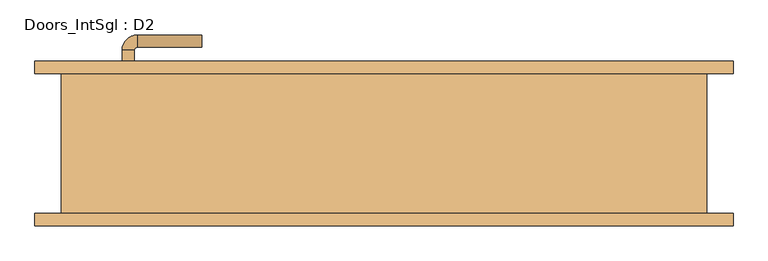
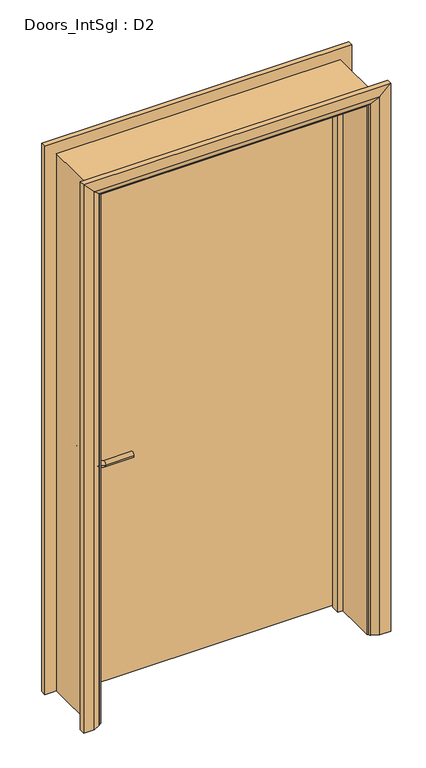
"""IFC4 building model written with IfcOpenShell, lengths in millimetres: door geometry, Doors_IntSgl : D2."""

from ifc_helpers import new_model, si_unit, point, frame, frame_2d, origin, place, context, project, spatial, polyline, circle_curve, ellipse_curve, trimmed, segment, composite_curve, outline, extrude, faceted_brep, source, transform, mapped, element, save
from ifc_brep_helpers import plane_surface, cylinder_surface, revolved_surface, advanced_brep


def doors_intsgl_d2_1027b9ee(model_context):
    return source(origin(), model_context, "Body", "SolidModel", [
        advanced_brep(
        [(-426.4, 68.3, 900.0), (-406.4, 68.3, 900.0), (-406.4, 38.3, 900.0), (-426.4, 38.3, 900.0), (-401.4, 33.3, 900.0), (-401.4, 13.3, 900.0), (-296.4, 13.3, 900.0), (-296.4, 33.3, 900.0)],
        [
            (0, 1, circle_curve(frame((-416.4, 68.3, 900.0), z_axis=(0.0, 1.0, 0.0), x_axis=(1.0, 0.0, 0.0)), 10.0)),
            (1, 0, circle_curve(frame((-416.4, 68.3, 900.0), z_axis=(0.0, 1.0, 0.0), x_axis=(1.0, 0.0, 0.0)), 10.0)),
            (1, 2),
            (2, 3, circle_curve(frame((-416.4, 38.3, 900.0), z_axis=(0.0, 1.0, 0.0), x_axis=(1.0, 0.0, 0.0)), 10.0)),
            (3, 0),
            (3, 2, circle_curve(frame((-416.4, 38.3, 900.0), z_axis=(0.0, 1.0, 0.0), x_axis=(1.0, 0.0, 0.0)), 10.0)),
            (4, 5, circle_curve(frame((-401.4, 23.3, 900.0), z_axis=(-1.0, 0.0, 0.0), x_axis=(0.0, 1.0, 0.0)), 10.0)),
            (5, 3, circle_curve(frame((-401.4, 38.3, 900.0), z_axis=(0.0, 0.0, -1.0), x_axis=(-1.0, 0.0, 0.0)), 25.0)),
            (2, 4, circle_curve(frame((-401.4, 38.3, 900.0), z_axis=(0.0, 0.0, 1.0), x_axis=(-1.0, 0.0, 0.0)), 5.0)),
            (5, 4, circle_curve(frame((-401.4, 23.3, 900.0), z_axis=(-1.0, 0.0, 0.0), x_axis=(0.0, 1.0, 0.0)), 10.0)),
            (6, 7, circle_curve(frame((-296.4, 23.3, 900.0), z_axis=(1.0, 0.0, 0.0), x_axis=(0.0, 1.0, 0.0)), 10.0)),
            (7, 6, circle_curve(frame((-296.4, 23.3, 900.0), z_axis=(1.0, 0.0, 0.0), x_axis=(0.0, 1.0, 0.0)), 10.0)),
            (4, 7),
            (6, 5),
        ],
        [
            plane_surface(frame((-416.4, 68.3, 900.0), z_axis=(0.0, 1.0, 0.0), x_axis=(0.0, 0.0, 1.0))),
            cylinder_surface(frame((-416.4, 68.3, 900.0), z_axis=(0.0, 1.0, 0.0), x_axis=(1.0, 0.0, 0.0)), 10.0),
            revolved_surface(trimmed(ellipse_curve(frame((-416.4, 38.3, 900.0), z_axis=(0.0, -1.0, 0.0), x_axis=(1.0, 0.0, 0.0)), 10.0, 10.0), [point((-426.4, 38.3, 900.0))], [point((-406.4, 38.3, 900.0))], True, "CARTESIAN"), (-401.4, 38.3, 900.0), (0.0, 0.0, -1.0)),
            revolved_surface(trimmed(ellipse_curve(frame((-416.4, 38.3, 900.0), z_axis=(0.0, -1.0, 0.0), x_axis=(1.0, 0.0, 0.0)), 10.0, 10.0), [point((-406.4, 38.3, 900.0))], [point((-426.4, 38.3, 900.0))], True, "CARTESIAN"), (-401.4, 38.3, 900.0), (0.0, 0.0, -1.0)),
            plane_surface(frame((-296.4, 23.3, 900.0), z_axis=(1.0, 0.0, 0.0), x_axis=(0.0, 0.0, 1.0))),
            cylinder_surface(frame((-401.4, 23.3, 900.0), z_axis=(-1.0, 0.0, 0.0), x_axis=(0.0, 1.0, 0.0)), 10.0),
        ],
        [
            (0, [[1, 2]]),
            (1, [[3, 4, 5, -2]]),
            (1, [[-5, 6, -3, -1]]),
            (2, [[7, 8, -4, 9]]),
            (3, [[10, -9, -6, -8]]),
            (4, [[11, 12]]),
            (5, [[13, -11, 14, -7]]),
            (5, [[-14, -12, -13, -10]]),
        ],
    ),
        extrude(outline(composite_curve([segment(trimmed(circle_curve(frame_2d((900.0, -418.9)), 30.0), [point((900.0, -448.9))], [point((900.0, -388.9))], False, "CARTESIAN"), True, "CONTINUOUS"), segment(trimmed(circle_curve(frame_2d((900.0, -418.9)), 30.0), [point((900.0, -388.9))], [point((900.0, -448.9))], False, "CARTESIAN"), True, "CONTINUOUS")], self_intersect=False)), frame((0.0, 68.3, 0.0), z_axis=(0.0, 1.0, 0.0), x_axis=(0.0, 0.0, 1.0)), (0.0, 0.0, 1.0), 8.0),
        advanced_brep(
        [(-426.4, 122.3, 900.0), (-406.4, 122.3, 900.0), (-426.4, 152.3, 900.0), (-406.4, 152.3, 900.0), (-401.4, 157.3, 900.0), (-401.4, 177.3, 900.0), (-296.4, 177.3, 900.0), (-296.4, 157.3, 900.0)],
        [
            (0, 1, circle_curve(frame((-416.4, 122.3, 900.0), z_axis=(0.0, -1.0, 0.0), x_axis=(1.0, 0.0, 0.0)), 10.0)),
            (1, 0, circle_curve(frame((-416.4, 122.3, 900.0), z_axis=(0.0, -1.0, 0.0), x_axis=(1.0, 0.0, 0.0)), 10.0)),
            (0, 2),
            (2, 3, circle_curve(frame((-416.4, 152.3, 900.0), z_axis=(0.0, -1.0, 0.0), x_axis=(1.0, 0.0, 0.0)), 10.0)),
            (3, 1),
            (3, 2, circle_curve(frame((-416.4, 152.3, 900.0), z_axis=(0.0, -1.0, 0.0), x_axis=(1.0, 0.0, 0.0)), 10.0)),
            (4, 3, circle_curve(frame((-401.4, 152.3, 900.0), z_axis=(0.0, 0.0, 1.0), x_axis=(-1.0, 0.0, 0.0)), 5.0)),
            (2, 5, circle_curve(frame((-401.4, 152.3, 900.0), z_axis=(0.0, 0.0, -1.0), x_axis=(-1.0, 0.0, 0.0)), 25.0)),
            (5, 4, circle_curve(frame((-401.4, 167.3, 900.0), z_axis=(-1.0, 0.0, 0.0), x_axis=(0.0, -1.0, 0.0)), 10.0)),
            (4, 5, circle_curve(frame((-401.4, 167.3, 900.0), z_axis=(-1.0, 0.0, 0.0), x_axis=(0.0, -1.0, 0.0)), 10.0)),
            (6, 7, circle_curve(frame((-296.4, 167.3, 900.0), z_axis=(1.0, 0.0, 0.0), x_axis=(0.0, -1.0, 0.0)), 10.0)),
            (7, 6, circle_curve(frame((-296.4, 167.3, 900.0), z_axis=(1.0, 0.0, 0.0), x_axis=(0.0, -1.0, 0.0)), 10.0)),
            (5, 6),
            (7, 4),
        ],
        [
            plane_surface(frame((-416.4, 122.3, 900.0), z_axis=(0.0, -1.0, 0.0), x_axis=(0.0, 0.0, 1.0))),
            cylinder_surface(frame((-416.4, 122.3, 900.0), z_axis=(0.0, -1.0, 0.0), x_axis=(1.0, 0.0, 0.0)), 10.0),
            revolved_surface(trimmed(ellipse_curve(frame((-416.4, 152.3, 900.0), z_axis=(0.0, -1.0, 0.0), x_axis=(1.0, 0.0, 0.0)), 10.0, 10.0), [point((-426.4, 152.3, 900.0))], [point((-406.4, 152.3, 900.0))], True, "CARTESIAN"), (-401.4, 152.3, 900.0), (0.0, 0.0, -1.0)),
            revolved_surface(trimmed(ellipse_curve(frame((-416.4, 152.3, 900.0), z_axis=(0.0, -1.0, 0.0), x_axis=(1.0, 0.0, 0.0)), 10.0, 10.0), [point((-406.4, 152.3, 900.0))], [point((-426.4, 152.3, 900.0))], True, "CARTESIAN"), (-401.4, 152.3, 900.0), (0.0, 0.0, -1.0)),
            plane_surface(frame((-296.4, 167.3, 900.0), z_axis=(1.0, 0.0, 0.0), x_axis=(0.0, 0.0, 1.0))),
            cylinder_surface(frame((-401.4, 167.3, 900.0), z_axis=(-1.0, 0.0, 0.0), x_axis=(0.0, -1.0, 0.0)), 10.0),
        ],
        [
            (0, [[1, 2]]),
            (1, [[-1, 3, 4, 5]]),
            (1, [[-2, -5, 6, -3]]),
            (2, [[7, -4, 8, 9]]),
            (3, [[-8, -6, -7, 10]]),
            (4, [[11, 12]]),
            (5, [[-9, 13, -12, 14]]),
            (5, [[-10, -14, -11, -13]]),
        ],
    ),
        extrude(outline(composite_curve([segment(trimmed(circle_curve(frame_2d((900.0, -418.9)), 30.0), [point((900.0, -448.9))], [point((900.0, -388.9))], False, "CARTESIAN"), True, "CONTINUOUS"), segment(trimmed(circle_curve(frame_2d((900.0, -418.9)), 30.0), [point((900.0, -388.9))], [point((900.0, -448.9))], False, "CARTESIAN"), True, "CONTINUOUS")], self_intersect=False)), frame((0.0, 114.3, 0.0), z_axis=(0.0, 1.0, 0.0), x_axis=(0.0, 0.0, 1.0)), (0.0, 0.0, 1.0), 8.0),
        extrude(outline(polyline([(491.4, 76.3), (-491.4, 76.3), (-491.4, 114.3), (491.4, 114.3), (491.4, 76.3)])), frame((0.0, 0.0, 8.0), z_axis=(0.0, 0.0, 1.0), x_axis=(1.0, 0.0, 0.0)), (0.0, 0.0, 1.0), 2060.0),
        advanced_brep(
        [(568.4, 134.3, 0.0), (568.4, 114.3, 0.0), (498.4, 114.3, 0.0), (502.4, 120.3, 0.0), (528.4, 134.3, 0.0), (568.4, 134.3, 2145.0), (568.4, 114.3, 2145.0), (-568.4, 114.3, 2145.0), (-568.4, 114.3, 0.0), (-498.4, 114.3, 0.0), (-498.4, 114.3, 2075.0), (498.4, 114.3, 2075.0), (502.4, 120.3, 2079.0), (528.4, 134.3, 2105.0), (-528.4, 134.3, 2105.0), (-528.4, 134.3, 0.0), (-568.4, 134.3, 0.0), (-568.4, 134.3, 2145.0), (-502.4, 120.3, 0.0), (-502.4, 120.3, 2079.0)],
        [
            (0, 1),
            (1, 2),
            (2, 3, circle_curve(frame((506.4, 113.3, 0.0), z_axis=(0.0, 0.0, -1.0), x_axis=(1.0, 0.0, 0.0)), 8.0622577)),
            (3, 4),
            (4, 0),
            (0, 5),
            (5, 6),
            (6, 1),
            (6, 7),
            (7, 8),
            (8, 9),
            (9, 10),
            (10, 11),
            (11, 2),
            (11, 12, ellipse_curve(frame((506.4, 113.3, 2083.0), z_axis=(0.7071067811865475, 0.0, -0.7071067811865475), x_axis=(-0.7071067811865474, 0.0, -0.7071067811865476)), 11.4017543, 8.0622577)),
            (12, 3),
            (12, 13),
            (13, 4),
            (13, 14),
            (14, 15),
            (15, 16),
            (16, 17),
            (17, 5),
            (7, 17),
            (16, 8),
            (15, 18),
            (18, 9, circle_curve(frame((-506.4, 113.3, 0.0), z_axis=(0.0, 0.0, -1.0), x_axis=(-1.0, 0.0, 0.0)), 8.0622577)),
            (19, 10, ellipse_curve(frame((-506.4, 113.3, 2083.0), z_axis=(-0.7071067811865475, 0.0, -0.7071067811865475), x_axis=(-0.7071067811865474, 0.0, 0.7071067811865476)), 11.4017543, 8.0622577)),
            (18, 19),
            (14, 19),
            (19, 12),
        ],
        [
            plane_surface(frame((498.4, 114.3, 0.0), z_axis=(0.0, 0.0, -1.0), x_axis=(0.0, -1.0, 0.0))),
            plane_surface(frame((568.4, 134.3, 0.0), z_axis=(1.0, 0.0, 0.0), x_axis=(0.0, 0.0, 1.0))),
            plane_surface(frame((568.4, 114.3, 0.0), z_axis=(0.0, -1.0, 0.0), x_axis=(0.0, 0.0, 1.0))),
            cylinder_surface(frame((506.4, 113.3, 0.0), z_axis=(0.0, 0.0, -1.0), x_axis=(1.0, 0.0, 0.0)), 8.0622577),
            plane_surface(frame((502.4, 120.3, 0.0), z_axis=(-0.4740998230350126, 0.880471099922178, 0.0), x_axis=(0.0, 0.0, 1.0))),
            plane_surface(frame((528.4, 134.3, 0.0), z_axis=(0.0, 1.0, 0.0), x_axis=(0.0, 0.0, 1.0))),
            plane_surface(frame((-568.4, 134.3, 2145.0), z_axis=(-1.0, 0.0, 0.0), x_axis=(0.0, 0.0, -1.0))),
            plane_surface(frame((-498.4, 114.3, 0.0), z_axis=(0.0, 0.0, -1.0), x_axis=(0.0, -1.0, 0.0))),
            cylinder_surface(frame((-506.4, 113.3, 2075.0), z_axis=(0.0, 0.0, 1.0), x_axis=(-1.0, 0.0, 0.0)), 8.0622577),
            plane_surface(frame((-502.4, 120.3, 2079.0), z_axis=(0.47409982303501824, 0.8804710999221749, 0.0), x_axis=(0.0, 0.0, -1.0))),
            plane_surface(frame((568.4, 134.3, 2145.0), z_axis=(0.0, 0.0, 1.0), x_axis=(-1.0, 0.0, 0.0))),
            cylinder_surface(frame((498.4, 113.3, 2083.0), z_axis=(1.0, 0.0, 0.0), x_axis=(0.0, 0.0, 1.0)), 8.0622577),
            plane_surface(frame((502.4, 120.3, 2079.0), z_axis=(0.0, 0.8804710999221764, -0.4740998230350154), x_axis=(-1.0, 0.0, 0.0))),
        ],
        [
            (0, [[1, 2, 3, 4, 5]]),
            (1, [[-1, 6, 7, 8]]),
            (2, [[-2, -8, 9, 10, 11, 12, 13, 14]]),
            (3, [[-3, -14, 15, 16]]),
            (4, [[-4, -16, 17, 18]]),
            (5, [[-5, -18, 19, 20, 21, 22, 23, -6]]),
            (6, [[24, -22, 25, -10]]),
            (7, [[-21, 26, 27, -11, -25]]),
            (8, [[28, -12, -27, 29]]),
            (9, [[30, -29, -26, -20]]),
            (10, [[-7, -23, -24, -9]]),
            (11, [[-15, -13, -28, 31]]),
            (12, [[-17, -31, -30, -19]]),
        ],
    ),
        extrude(outline(polyline([(0.0, -493.4), (0.0, -474.4), (2051.0, -474.4), (2051.0, 474.4), (0.0, 474.4), (0.0, 493.4), (2070.0, 493.4), (2070.0, -493.4), (0.0, -493.4)])), frame((0.0, 42.3, 0.0), z_axis=(0.0, 1.0, 0.0), x_axis=(0.0, 0.0, 1.0)), (0.0, 0.0, 1.0), 32.0),
        advanced_brep(
        [(-568.4, -134.3, 0.0), (-568.4, -114.3, 0.0), (-498.4, -114.3, 0.0), (-502.4, -120.3, 0.0), (-528.4, -134.3, 0.0), (-568.4, -134.3, 2145.0), (-568.4, -114.3, 2145.0), (-498.4, -114.3, 2075.0), (-502.4, -120.3, 2079.0), (-528.4, -134.3, 2105.0), (568.4, -134.3, 0.0), (528.4, -134.3, 0.0), (502.4, -120.3, 0.0), (498.4, -114.3, 0.0), (568.4, -114.3, 0.0), (568.4, -134.3, 2145.0), (528.4, -134.3, 2105.0), (502.4, -120.3, 2079.0), (498.4, -114.3, 2075.0), (568.4, -114.3, 2145.0)],
        [
            (0, 1),
            (1, 2),
            (2, 3, circle_curve(frame((-506.4, -113.3, 0.0), z_axis=(0.0, 0.0, -1.0), x_axis=(-1.0, 0.0, 0.0)), 8.0622577)),
            (3, 4),
            (4, 0),
            (0, 5),
            (5, 6),
            (6, 1),
            (6, 7),
            (7, 2),
            (7, 8, ellipse_curve(frame((-506.4, -113.3, 2083.0), z_axis=(-0.7071067811865475, 0.0, -0.7071067811865475), x_axis=(0.7071067811865474, 0.0, -0.7071067811865476)), 11.4017543, 8.0622577)),
            (8, 3),
            (8, 9),
            (9, 4),
            (9, 5),
            (10, 11),
            (11, 12),
            (12, 13, circle_curve(frame((506.4, -113.3, 0.0), z_axis=(0.0, 0.0, -1.0), x_axis=(1.0, 0.0, 0.0)), 8.0622577)),
            (13, 14),
            (14, 10),
            (15, 16),
            (16, 11),
            (10, 15),
            (16, 17),
            (17, 12),
            (17, 18, ellipse_curve(frame((506.4, -113.3, 2083.0), z_axis=(0.7071067811865475, 0.0, -0.7071067811865475), x_axis=(0.7071067811865474, 0.0, 0.7071067811865476)), 11.4017543, 8.0622577)),
            (18, 13),
            (18, 19),
            (19, 14),
            (19, 15),
            (5, 15),
            (19, 6),
            (18, 7),
            (17, 8),
            (16, 9),
        ],
        [
            plane_surface(frame((-498.4, -187.1010989, 0.0), z_axis=(0.0, 0.0, -1.0), x_axis=(1.0, 0.0, 0.0))),
            plane_surface(frame((-568.4, -134.3, 0.0), z_axis=(-1.0, 0.0, 0.0), x_axis=(0.0, 0.0, 1.0))),
            plane_surface(frame((-568.4, -114.3, 0.0), z_axis=(0.0, 1.0, 0.0), x_axis=(0.0, 0.0, 1.0))),
            cylinder_surface(frame((-506.4, -113.3, 0.0), z_axis=(0.0, 0.0, -1.0), x_axis=(-1.0, 0.0, 0.0)), 8.0622577),
            plane_surface(frame((-502.4, -120.3, 0.0), z_axis=(0.4740998230350183, -0.8804710999221749, 0.0), x_axis=(0.0, 0.0, 1.0))),
            plane_surface(frame((-528.4, -134.3, 0.0), z_axis=(0.0, -1.0, 0.0), x_axis=(0.0, 0.0, 1.0))),
            plane_surface(frame((498.4, -187.1010989, 0.0), z_axis=(0.0, 0.0, -1.0), x_axis=(-1.0, 0.0, 0.0))),
            plane_surface(frame((528.4, -134.3, 2105.0), z_axis=(0.0, -1.0, 0.0), x_axis=(0.0, 0.0, -1.0))),
            plane_surface(frame((502.4, -120.3, 2079.0), z_axis=(-0.4740998230350183, -0.8804710999221749, 0.0), x_axis=(0.0, 0.0, -1.0))),
            cylinder_surface(frame((506.4, -113.3, 2075.0), z_axis=(0.0, 0.0, 1.0), x_axis=(1.0, 0.0, 0.0)), 8.0622577),
            plane_surface(frame((568.4, -114.3, 2145.0), z_axis=(0.0, 1.0, 0.0), x_axis=(0.0, 0.0, -1.0))),
            plane_surface(frame((568.4, -134.3, 2145.0), z_axis=(1.0, 0.0, 0.0), x_axis=(0.0, 0.0, -1.0))),
            plane_surface(frame((-568.4, -134.3, 2145.0), z_axis=(0.0, 0.0, 1.0), x_axis=(1.0, 0.0, 0.0))),
            plane_surface(frame((-568.4, -114.3, 2145.0), z_axis=(0.0, 1.0, 0.0), x_axis=(1.0, 0.0, 0.0))),
            cylinder_surface(frame((-498.4, -113.3, 2083.0), z_axis=(-1.0, 0.0, 0.0), x_axis=(0.0, 0.0, 1.0)), 8.0622577),
            plane_surface(frame((-502.4, -120.3, 2079.0), z_axis=(0.0, -0.8804710999221749, -0.4740998230350183), x_axis=(1.0, 0.0, 0.0))),
            plane_surface(frame((-528.4, -134.3, 2105.0), z_axis=(0.0, -1.0, 0.0), x_axis=(1.0, 0.0, 0.0))),
        ],
        [
            (0, [[1, 2, 3, 4, 5]]),
            (1, [[-1, 6, 7, 8]]),
            (2, [[-2, -8, 9, 10]]),
            (3, [[-3, -10, 11, 12]]),
            (4, [[-4, -12, 13, 14]]),
            (5, [[-5, -14, 15, -6]]),
            (6, [[16, 17, 18, 19, 20]]),
            (7, [[21, 22, -16, 23]]),
            (8, [[24, 25, -17, -22]]),
            (9, [[26, 27, -18, -25]]),
            (10, [[28, 29, -19, -27]]),
            (11, [[30, -23, -20, -29]]),
            (12, [[-7, 31, -30, 32]]),
            (13, [[-9, -32, -28, 33]]),
            (14, [[-11, -33, -26, 34]]),
            (15, [[-13, -34, -24, 35]]),
            (16, [[-15, -35, -21, -31]]),
        ],
    ),
        faceted_brep([(-493.4, 114.3, 0.0), (-493.4, -114.3, 0.0), (-525.4, -114.3, 0.0), (-525.4, 114.3, 0.0), (-493.4, 114.3, 2070.0), (-493.4, -114.3, 2070.0), (-525.4, -114.3, 2102.0), (-525.4, 114.3, 2102.0), (493.4, 114.3, 0.0), (525.4, 114.3, 0.0), (525.4, -114.3, 0.0), (493.4, -114.3, 0.0), (493.4, 114.3, 2070.0), (525.4, 114.3, 2102.0), (525.4, -114.3, 2102.0), (493.4, -114.3, 2070.0)], [[[0, 1, 2, 3]], [[1, 0, 4, 5]], [[2, 1, 5, 6]], [[3, 2, 6, 7]], [[0, 3, 7, 4]], [[8, 9, 10, 11]], [[12, 13, 9, 8]], [[13, 14, 10, 9]], [[14, 15, 11, 10]], [[15, 12, 8, 11]], [[5, 4, 12, 15]], [[6, 5, 15, 14]], [[7, 6, 14, 13]], [[4, 7, 13, 12]]]),
    ])


if __name__ == "__main__":
    model = new_model("IFC4")
    model_context = context("Model", 3, world=origin())
    ifc_project = project(units=[si_unit("LENGTHUNIT", "METRE", prefix="MILLI")], contexts=[model_context])
    site = spatial("IfcSite", under=ifc_project)
    building = spatial("IfcBuilding", under=site)
    placement = place(None, origin())
    doors_intsgl_d2_shape = doors_intsgl_d2_1027b9ee(model_context)
    element("IfcDoor", 1, ObjectType="Doors_IntSgl : D2", at=placement, inside=building, context=model_context, shape_type="MappedRepresentation", body=[
        mapped(doors_intsgl_d2_shape, transform((0.0, 0.0, 0.0), x_axis=(1.0, 0.0, 0.0), y_axis=(0.0, 1.0, 0.0), z_axis=(0.0, 0.0, 1.0))),
    ])
    save(model, "model.ifc")

# Revit data of these elements
# Type "Doors_IntSgl : D2"
#   Type Mark = "49"
#   Type Comments = "Internal Single"
#   Operation = "SingleSwingRight"
#   Manufacturer = "Revit"
#   Keynote = "L20"
#   Description = "Internal Single Door"
#   Analytic Construction = "Metal"
#   UnderCut = 0.026247 ft
#   Tolerance = 0.006562 ft
#   Thickness = 0.124672 ft
#   Thermal Resistance (R) = 0.270117 (m²·K)/W
#   Structural Tolerance = 0.026247 ft
#   StopDepth = 0.104987 ft
#   Stop Thickness = 0.062336 ft
#   Rough Width = 3.5 ft
#   Rough Height = 6.922572 ft
#   Height to Top Lock Rail = 3.28084 ft
#   Heat Transfer Coefficient (U) = 3.7021 W/(m²·K)
#   Handle Z Distance = 2.952756 ft
#   Handle X Distance = 0.246063 ft
#   Frame Thickness = 0.104987 ft
#   Door Panel Width = 3.224409 ft
#   Door Panel Thickness = 0.124672 ft
#   Door Panel Offset = 0.0 ft
#   Height = 6.922572 ft
#   Width = 3.5 ft
#   Door Panel Height = 6.75853 ft
#   Architrave Setback = 0.016404 ft
#   Vis - Ironmongery = yes
#   Material Ironmongery = Door - Handle
#   Material Frame = Door - Frame/Mullion (1)
#   Material Door = Door - Panel
#   Material Architrave = Door - Architrave
#   Visual Light Transmittance = 0
#   Solar Heat Gain Coefficient = 0
#   Function = (empty or 0)
#   Wall Closure = (empty or 0)
# Element 1 (IfcDoor, "Doors_IntSgl : D2")
#   Materials on its faces: "Door - Architrave", "Door - Handle", "Door - Frame/Mullion (1)", "Door - Panel"
# Materials
#   "Door - Handle": colour RGB 0 0 0, transparency 0, Keynote = "P21", Cost = 0
#   "Door - Frame/Mullion (1)": class "Wood", colour RGB 212 179 113, transparency 0, Keynote = "L20", Cost = 0
#   "Door - Panel": class "Wood", colour RGB 210 159 95, transparency 0, Keynote = "L20", Cost = 0
#   "Door - Architrave": class "Wood", colour RGB 154 90 5, transparency 0, Keynote = "P20", Cost = 0
